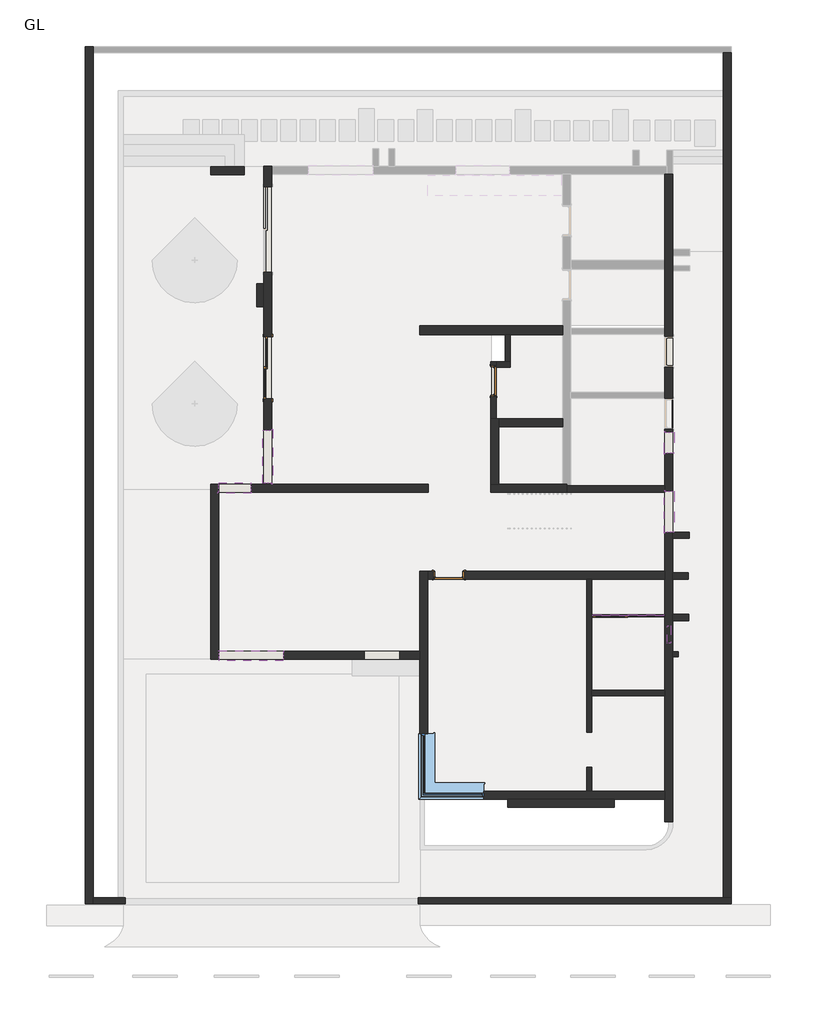
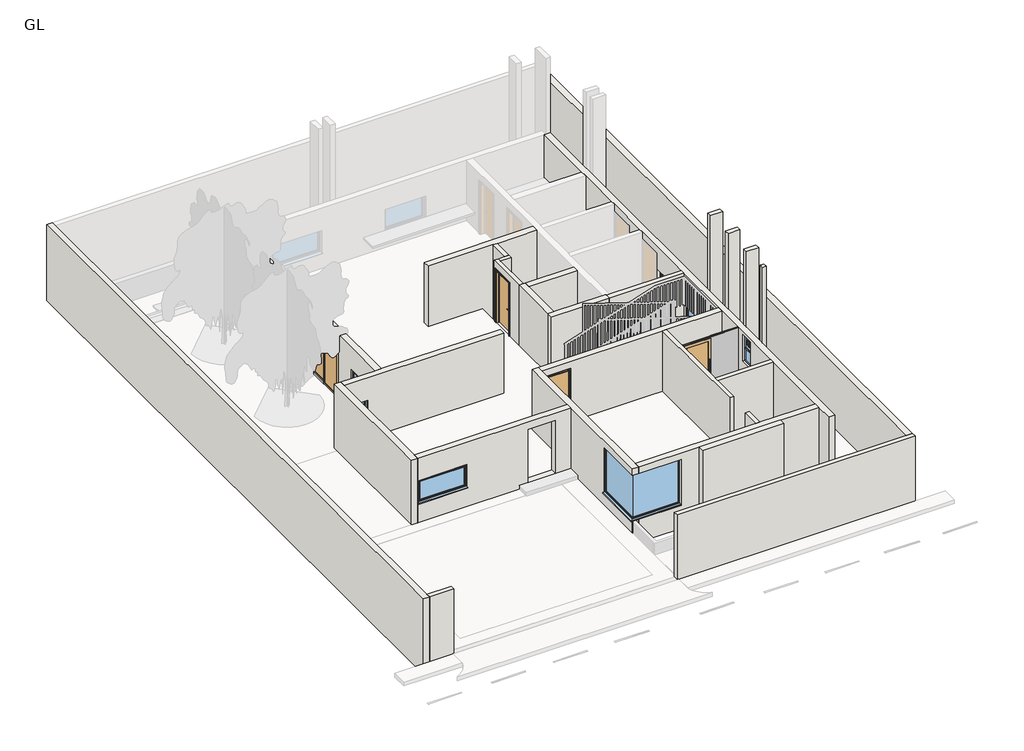
# One storey, part 1 of 6: 30 walls, 7 members, 7 windows, 4 doors, 1 plate.
"""IFC4 building model written with IfcOpenShell, lengths in millimetres."""

from ifc_helpers import new_model, si_unit, point, frame, frame_2d, origin, origin_with_axes, place, context, project, spatial, polyline, circle_curve, ellipse_curve, trimmed, segment, composite_curve, outline, extrude, faceted_brep, transform, mapped, element, save
from ifc_brep_helpers import plane_surface, cylinder_surface, revolved_surface, advanced_brep
from components import door_510b0506, door_61435f0d, door_526ed47c, doors_sgl_glass_1_glass_panel_12mm_thickness_6ba6481b, rectangular_mullion_30mm_square_d725415c, rectangular_mullion_30mm_square_ff288ed3, rectangular_mullion_30mm_square_6919c9ce, system_panel_glazed_4603f3ec, windows_corner_1829x1829mm_2_98ac2af9, windows_sgl_plain_2_8d1346b0, windows_sgl_plain_3_28d0678b, window_6a333e19, windows_sgl_plain_5_79f17ecf, windows_sgl_plain_6_3dcb7f7b

model = new_model("IFC4")

# Units and contexts
model_context = context("Model", 3, world=origin())
ifc_project = project(units=[si_unit("LENGTHUNIT", "METRE", prefix="MILLI")], contexts=[model_context])

# Site, building, storey
site = spatial("IfcSite", under=ifc_project)
building = spatial("IfcBuilding", under=site)
storey = spatial("IfcBuildingStorey", under=building, Name="GL", Elevation=0.0)

# Doors
placement = place(None, origin())
door_shape = door_510b0506(model_context)
element("IfcDoor", 1, ObjectType="5'10\"", at=placement, inside=storey, context=model_context, shape_type="MappedRepresentation", body=[
    mapped(door_shape, transform((-46875.1786333, 21413.0648243, 449.9570313), x_axis=(0.0, 1.0, 0.0), y_axis=(-1.0, 0.0, 0.0), z_axis=(0.0, 0.0, 1.0))),
])
door_2_shape = door_61435f0d(model_context)
element("IfcDoor", 2, ObjectType="Doors_IntSgl : 2'11\"", at=placement, inside=storey, context=model_context, shape_type="MappedRepresentation", body=[
    mapped(door_2_shape, transform((-41829.89796, 15488.6041063, 580.01875), x_axis=(-1.0, 0.0, 0.0), y_axis=(0.0, -1.0, 0.0), z_axis=(0.0, 0.0, 1.0))),
])
door_3_shape = door_526ed47c(model_context)
element("IfcDoor", 3, ObjectType="Doors_IntSgl : 2'11\"", at=placement, inside=storey, context=model_context, shape_type="MappedRepresentation", body=[
    mapped(door_3_shape, transform((-40553.54796, 21038.5041063, 589.9546875), x_axis=(0.0, 1.0, 0.0), y_axis=(-1.0, 0.0, 0.0), z_axis=(0.0, 0.0, 1.0))),
])
doors_sgl_glass_1_glass_panel_12mm_thickness_shape = doors_sgl_glass_1_glass_panel_12mm_thickness_6ba6481b(model_context)
element("IfcDoor", 4, ObjectType="Doors_Sgl_Glass_1 : Glass_Panel-12mm_Thickness", at=placement, inside=storey, context=model_context, shape_type="MappedRepresentation", body=[
    mapped(doors_sgl_glass_1_glass_panel_12mm_thickness_shape, transform((-37210.5680043, 14342.1489352, 629.9757812), x_axis=(-1.0, 0.0, 0.0), y_axis=(0.0, -1.0, 0.0), z_axis=(0.0, 0.0, 1.0))),
])

# Members
rectangular_mullion_30mm_square_shape = rectangular_mullion_30mm_square_d725415c(model_context)
element("IfcMember", 5, ObjectType="Rectangular Mullion : 30mm_Square", at=placement, inside=storey, context=model_context, shape_type="MappedRepresentation", body=[
    mapped(rectangular_mullion_30mm_square_shape, transform((-37710.3080191, 14342.1489352, 3000.0), x_axis=(0.0, 0.0, 1.0), y_axis=(0.0, 1.0, 0.0), z_axis=(-1.0, 0.0, 0.0))),
])
element("IfcMember", 6, ObjectType="Rectangular Mullion : 30mm_Square", at=placement, inside=storey, context=model_context, shape_type="MappedRepresentation", body=[
    mapped(rectangular_mullion_30mm_square_shape, transform((-36680.8279896, 14342.1489352, 3000.0), x_axis=(0.0, 0.0, 1.0), y_axis=(0.0, 1.0, 0.0), z_axis=(-1.0, 0.0, 0.0))),
])
element("IfcMember", 7, ObjectType="Rectangular Mullion : 30mm_Square", at=placement, inside=storey, context=model_context, shape_type="MappedRepresentation", body=[
    mapped(rectangular_mullion_30mm_square_shape, transform((-35681.34796, 14342.1489352, 599.9757812), x_axis=(0.0, 0.0, -1.0), y_axis=(0.0, 1.0, 0.0), z_axis=(1.0, 0.0, 0.0))),
])
element("IfcMember", 8, ObjectType="Rectangular Mullion : 30mm_Square", at=placement, inside=storey, context=model_context, shape_type="MappedRepresentation", body=[
    mapped(rectangular_mullion_30mm_square_shape, transform((-36710.8279896, 14342.1489352, 599.9757812), x_axis=(0.0, 0.0, -1.0), y_axis=(0.0, 1.0, 0.0), z_axis=(1.0, 0.0, 0.0))),
])
rectangular_mullion_30mm_square_2_shape = rectangular_mullion_30mm_square_ff288ed3(model_context)
element("IfcMember", 9, ObjectType="Rectangular Mullion : 30mm_Square", at=placement, inside=storey, context=model_context, shape_type="MappedRepresentation", body=[
    mapped(rectangular_mullion_30mm_square_2_shape, transform((-36695.8279896, 14342.1489352, 599.9757812), x_axis=(-1.0, 0.0, 0.0), y_axis=(0.0, 1.0, 0.0), z_axis=(0.0, 0.0, -1.0))),
])
rectangular_mullion_30mm_square_3_shape = rectangular_mullion_30mm_square_6919c9ce(model_context)
element("IfcMember", 10, ObjectType="Rectangular Mullion : 30mm_Square", at=placement, inside=storey, context=model_context, shape_type="MappedRepresentation", body=[
    mapped(rectangular_mullion_30mm_square_3_shape, transform((-35651.34796, 14342.1489352, 3000.0), x_axis=(1.0, 0.0, 0.0), y_axis=(0.0, 1.0, 0.0), z_axis=(0.0, 0.0, 1.0))),
])
element("IfcMember", 11, ObjectType="Rectangular Mullion : 30mm_Square", at=placement, inside=storey, context=model_context, shape_type="MappedRepresentation", body=[
    mapped(rectangular_mullion_30mm_square_3_shape, transform((-37740.3080191, 14342.1489352, 599.9757812), x_axis=(-1.0, 0.0, 0.0), y_axis=(0.0, 1.0, 0.0), z_axis=(0.0, 0.0, -1.0))),
])

# Plate
system_panel_glazed_shape = system_panel_glazed_4603f3ec(model_context)
element("IfcPlate", 12, ObjectType="System Panel : Glazed", at=placement, inside=storey, context=model_context, shape_type="MappedRepresentation", body=[
    mapped(system_panel_glazed_shape, transform((-36173.5879748, 14342.1489352, 599.9757812), x_axis=(-1.0, 0.0, 0.0), y_axis=(0.0, -1.0, 0.0), z_axis=(0.0, 0.0, 1.0))),
])

# Walls
element("IfcWall", 13, ObjectType="6\" WALL", at=placement, inside=storey, context=model_context, shape_type="SweptSolid", body=[
    extrude(outline(polyline([(-37740.3080191, 9995.8541063), (-37740.3080191, 9303.7041063), (-37892.7080191, 9303.7041063), (-37892.7080191, 9995.8541063), (-37740.3080191, 9995.8541063)])), origin_with_axes(), (0.0, 0.0, 1.0), 3000.0),
])
element("IfcWall", 14, ObjectType="6\" WALL", at=placement, inside=storey, context=model_context, shape_type="Brep", body=[
    faceted_brep([(-37740.3080191, 10999.1541063, 0.0), (-37740.3080191, 12046.9041063, 0.0), (-37740.3080191, 12199.3041063, 0.0), (-37740.3080191, 15374.3041063, 0.0), (-37740.3080191, 15374.3041063, 3000.0), (-37740.3080191, 12199.3041063, 3000.0), (-37740.3080191, 12046.9041063, 3000.0), (-37740.3080191, 10999.1541063, 3000.0), (-37892.7080191, 10999.1541063, 0.0), (-37892.7080191, 10999.1541063, 3000.0), (-37892.7080191, 15374.3041063, 3000.0), (-37892.7080191, 15374.3041063, 0.0)], [[[0, 1, 2, 3, 4, 5, 6, 7]], [[8, 9, 10, 11]], [[3, 2, 1, 0, 8, 11]], [[7, 6, 5, 4, 10, 9]], [[0, 7, 9, 8]], [[4, 3, 11, 10]]]),
])
element("IfcWall", 15, ObjectType="6\" WALL", at=placement, inside=storey, context=model_context, shape_type="Brep", body=[
    faceted_brep([(-40477.34796, 19959.0041063, 0.0), (-40477.34796, 21432.2041063, 0.0), (-40477.34796, 21584.6041063, 0.0), (-40477.34796, 21584.6041063, 3000.0), (-40477.34796, 21432.2041063, 3000.0), (-40477.34796, 19959.0041063, 3000.0), (-40477.34796, 21483.0041063, 2699.9546875), (-40477.34796, 21483.0041063, 589.9546875), (-40477.34796, 20594.0041063, 589.9546875), (-40477.34796, 20594.0041063, 2699.9546875), (-40629.74796, 21584.6041063, 0.0), (-40629.74796, 19959.0041063, 0.0), (-40629.74796, 19959.0041063, 3000.0), (-40629.74796, 21584.6041063, 3000.0), (-40629.74796, 21483.0041063, 589.9546875), (-40629.74796, 21483.0041063, 2699.9546875), (-40629.74796, 20594.0041063, 2699.9546875), (-40629.74796, 20594.0041063, 589.9546875)], [[[0, 1, 2, 3, 4, 5], [6, 7, 8, 9]], [[10, 11, 12, 13], [14, 15, 16, 17]], [[2, 1, 0, 11, 10]], [[5, 4, 3, 13, 12]], [[0, 5, 12, 11]], [[3, 2, 10, 13]], [[14, 7, 6, 15]], [[15, 6, 9, 16]], [[16, 9, 8, 17]], [[7, 14, 17, 8]]]),
])
element("IfcWall", 16, ObjectType="6\" WALL", at=placement, inside=storey, context=model_context, shape_type="Brep", body=[
    faceted_brep([(-40477.34796, 21432.2041063, 0.0), (-40070.94796, 21432.2041063, 0.0), (-40070.94796, 21432.2041063, 3000.0), (-40477.34796, 21432.2041063, 3000.0), (-40477.34796, 21584.6041063, 0.0), (-40477.34796, 21584.6041063, 3000.0), (-40223.34796, 21584.6041063, 3000.0), (-40070.94796, 21584.6041063, 3000.0), (-40070.94796, 21584.6041063, 0.0), (-40223.34796, 21584.6041063, 0.0)], [[[0, 1, 2, 3]], [[4, 5, 6, 7, 8, 9]], [[1, 0, 4, 9, 8]], [[3, 2, 7, 6, 5]], [[0, 3, 5, 4]], [[2, 1, 8, 7]]]),
])
element("IfcWall", 17, ObjectType="6\" WALL", at=placement, inside=storey, context=model_context, shape_type="SweptSolid", body=[
    extrude(outline(polyline([(-40070.94796, 22359.3041063), (-40070.94796, 21584.6041063), (-40223.34796, 21584.6041063), (-40223.34796, 22359.3041063), (-40070.94796, 22359.3041063)])), origin_with_axes(), (0.0, 0.0, 1.0), 3000.0),
])
element("IfcWall", 18, ObjectType="6\" WALL", at=placement, inside=storey, context=model_context, shape_type="SweptSolid", body=[
    extrude(outline(polyline([(-37740.3080191, 12199.3041063), (-35651.34796, 12199.3041063), (-35651.34796, 12046.9041063), (-37740.3080191, 12046.9041063), (-37740.3080191, 12199.3041063)])), origin_with_axes(), (0.0, 0.0, 1.0), 3000.0),
])
element("IfcWall", 19, ObjectType="6\" WALL", at=placement, inside=storey, context=model_context, shape_type="SweptSolid", body=[
    extrude(outline(polyline([(-35422.74796, 13303.4981698), (-35276.2981431, 13303.4981698), (-35276.2981431, 13151.0981698), (-35422.74796, 13151.0981698), (-35422.74796, 13303.4981698)])), origin_with_axes(), (0.0, 0.0, 1.0), 6000.0),
])
element("IfcWall", 20, ObjectType="7\" WALL", at=placement, inside=storey, context=model_context, shape_type="Brep", body=[
    faceted_brep([(-35651.34796, 18041.3041063, 0.0), (-38343.74796, 18041.3041063, 0.0), (-38458.04796, 18041.3041063, 0.0), (-38458.04796, 18041.3041063, 3000.0), (-38343.74796, 18041.3041063, 3000.0), (-35651.34796, 18041.3041063, 3000.0), (-35651.34796, 17863.5041063, 0.0), (-35651.34796, 17863.5041063, 3000.0), (-38458.04796, 17863.5041063, 3000.0), (-38458.04796, 17863.5041063, 0.0)], [[[0, 1, 2, 3, 4, 5]], [[6, 7, 8, 9]], [[2, 1, 0, 6, 9]], [[3, 2, 9, 8]], [[5, 4, 3, 8, 7]], [[0, 5, 7, 6]]]),
])
element("IfcWall", 21, ObjectType="7\" WALL", at=placement, inside=storey, context=model_context, shape_type="SweptSolid", body=[
    extrude(outline(polyline([(-51085.1791975, 6088.2065956), (-51999.5791975, 6088.2065956), (-51999.5791975, 6266.0065956), (-51085.1791975, 6266.0065956), (-51085.1791975, 6088.2065956)])), origin_with_axes(), (0.0, 0.0, 1.0), 3000.0),
])
element("IfcWall", 22, ObjectType="7\" WALL", at=placement, inside=storey, context=model_context, shape_type="Brep", body=[
    faceted_brep([(-42703.1791975, 6088.2065956, 0.0), (-33762.3791975, 6088.2065956, 0.0), (-33762.3791975, 6088.2065956, 3000.0), (-42703.1791975, 6088.2065956, 3000.0), (-42703.1791975, 6266.0065956, 0.0), (-42703.1791975, 6266.0065956, 3000.0), (-33990.9791975, 6266.0065956, 3000.0), (-33762.3791975, 6266.0065956, 3000.0), (-33762.3791975, 6266.0065956, 0.0), (-33990.9791975, 6266.0065956, 0.0)], [[[0, 1, 2, 3]], [[4, 5, 6, 7, 8, 9]], [[1, 0, 4, 9, 8]], [[3, 2, 7, 6, 5]], [[0, 3, 5, 4]], [[2, 1, 8, 7]]]),
])
element("IfcWall", 23, ObjectType="7\" WALL", at=placement, inside=storey, context=model_context, shape_type="SweptSolid", body=[
    extrude(outline(polyline([(-35422.74796, 14367.5489352), (-34966.0759444, 14367.5489352), (-34966.0759444, 14189.7489352), (-35422.74796, 14189.7489352), (-35422.74796, 14367.5489352)])), origin_with_axes(), (0.0, 0.0, 1.0), 6000.0),
])
element("IfcWall", 24, ObjectType="7\" WALL", at=placement, inside=storey, context=model_context, shape_type="SweptSolid", body=[
    extrude(outline(polyline([(-35422.74796, 15551.8272539), (-34982.9645404, 15551.8272539), (-34982.9645404, 15374.0272539), (-35422.74796, 15374.0272539), (-35422.74796, 15551.8272539)])), origin_with_axes(), (0.0, 0.0, 1.0), 6000.0),
])
element("IfcWall", 25, ObjectType="7\" WALL", at=placement, inside=storey, context=model_context, shape_type="SweptSolid", body=[
    extrude(outline(polyline([(-35422.74796, 16715.1290984), (-34962.7027512, 16715.1290984), (-34962.7027512, 16537.3290984), (-35422.74796, 16537.3290984), (-35422.74796, 16715.1290984)])), origin_with_axes(), (0.0, 0.0, 1.0), 6000.0),
])
element("IfcWall", 26, ObjectType="8\" WALL", at=placement, inside=storey, context=model_context, shape_type="SweptSolid", body=[
    extrude(outline(polyline([(-47318.6226721, 23155.7652167), (-47318.6226721, 23816.1652167), (-47115.4226721, 23816.1652167), (-47115.4226721, 23155.7652167), (-47318.6226721, 23155.7652167)])), origin_with_axes(), (0.0, 0.0, 1.0), 3000.0),
])
element("IfcWall", 27, ObjectType="9\" INNER WALL", at=placement, inside=storey, context=model_context, shape_type="Brep", body=[
    faceted_brep([(-48411.8786333, 18085.6648243, 0.0), (-48411.8786333, 18085.6648243, 1200.0), (-47497.4786333, 18085.6648243, 1200.0), (-47497.4786333, 18085.6648243, 2110.0), (-48411.8786333, 18085.6648243, 2110.0), (-48411.8786333, 18085.6648243, 3000.0), (-47116.4786333, 18085.6648243, 3000.0), (-46887.8786333, 18085.6648243, 3000.0), (-42417.4786333, 18085.6648243, 3000.0), (-42417.4786333, 18085.6648243, 0.0), (-46887.8786333, 18085.6648243, 0.0), (-47116.4786333, 18085.6648243, 0.0), (-47497.4786333, 17857.0648243, 1200.0), (-48411.8786333, 17857.0648243, 1200.0), (-48411.8786333, 17857.0648243, 0.0), (-42417.4786333, 17857.0648243, 0.0), (-42417.4786333, 17857.0648243, 3000.0), (-48411.8786333, 17857.0648243, 3000.0), (-48411.8786333, 17857.0648243, 2110.0), (-47497.4786333, 17857.0648243, 2110.0)], [[[0, 1, 2, 3, 4, 5, 6, 7, 8, 9, 10, 11]], [[12, 13, 14, 15, 16, 17, 18, 19]], [[0, 11, 10, 9, 15, 14]], [[8, 7, 6, 5, 17, 16]], [[9, 8, 16, 15]], [[18, 17, 5, 4]], [[14, 13, 1, 0]], [[2, 1, 13, 12]], [[3, 2, 12, 19]], [[4, 3, 19, 18]]]),
])
element("IfcWall", 28, ObjectType="9\" INNER WALL", at=placement, inside=storey, context=model_context, shape_type="Brep", body=[
    faceted_brep([(-48640.4786333, 18085.6648243, 0.0), (-48640.4786333, 13078.7799463, 0.0), (-48640.4786333, 13078.7799463, 3000.0), (-48640.4786333, 18085.6648243, 3000.0), (-48411.8786333, 18085.6648243, 0.0), (-48411.8786333, 18085.6648243, 3000.0), (-48411.8786333, 17857.0648243, 3000.0), (-48411.8786333, 13307.3799463, 3000.0), (-48411.8786333, 13078.7799463, 3000.0), (-48411.8786333, 13078.7799463, 0.0), (-48411.8786333, 13307.3799463, 0.0), (-48411.8786333, 17857.0648243, 0.0)], [[[0, 1, 2, 3]], [[4, 5, 6, 7, 8, 9, 10, 11]], [[1, 0, 4, 11, 10, 9]], [[3, 2, 8, 7, 6, 5]], [[0, 3, 5, 4]], [[2, 1, 9, 8]]]),
])
element("IfcWall", 29, ObjectType="9\" INNER WALL", at=placement, inside=storey, context=model_context, shape_type="Brep", body=[
    faceted_brep([(-46887.8786333, 18085.6648243, 0.0), (-46887.8786333, 26943.9148243, 0.0), (-46887.8786333, 27172.5148243, 0.0), (-46887.8786333, 27172.5148243, 3000.0), (-46887.8786333, 26943.9148243, 3000.0), (-46887.8786333, 18085.6648243, 3000.0), (-46887.8786333, 18111.0648243, 2110.0), (-46887.8786333, 19635.0648243, 2110.0), (-46887.8786333, 19635.0648243, 1200.0), (-46887.8786333, 18111.0648243, 1200.0), (-46887.8786333, 20524.0648243, 2583.9570312), (-46887.8786333, 22302.0648243, 2583.9570312), (-46887.8786333, 22302.0648243, 449.9570312), (-46887.8786333, 20524.0648243, 449.9570313), (-46887.8786333, 24149.9148243, 2583.9570312), (-46887.8786333, 26588.3148243, 2583.9570312), (-46887.8786333, 26588.3148243, 449.9570312), (-46887.8786333, 24149.9148243, 449.9570313), (-47116.4786333, 18085.6648243, 0.0), (-47116.4786333, 18085.6648243, 3000.0), (-47116.4786333, 27172.5148243, 3000.0), (-47116.4786333, 27172.5148243, 0.0), (-47116.4786333, 18111.0648243, 2110.0), (-47116.4786333, 18111.0648243, 1200.0), (-47116.4786333, 19635.0648243, 1200.0), (-47116.4786333, 19635.0648243, 2110.0), (-47116.4786333, 20524.0648243, 2583.9570312), (-47116.4786333, 20524.0648243, 449.9570313), (-47116.4786333, 22302.0648243, 449.9570313), (-47116.4786333, 22302.0648243, 2583.9570312), (-47116.4786333, 24149.9148243, 2583.9570312), (-47116.4786333, 24149.9148243, 449.9570313), (-47116.4786333, 26588.3148243, 449.9570313), (-47116.4786333, 26588.3148243, 2583.9570312)], [[[0, 1, 2, 3, 4, 5], [6, 7, 8, 9], [10, 11, 12, 13], [14, 15, 16, 17]], [[18, 19, 20, 21], [22, 23, 24, 25], [26, 27, 28, 29], [30, 31, 32, 33]], [[2, 1, 0, 18, 21]], [[5, 4, 3, 20, 19]], [[0, 5, 19, 18]], [[3, 2, 21, 20]], [[23, 22, 6, 9]], [[24, 23, 9, 8]], [[25, 24, 8, 7]], [[22, 25, 7, 6]], [[27, 26, 10, 13]], [[28, 27, 13, 12]], [[29, 28, 12, 11]], [[26, 29, 11, 10]], [[31, 30, 14, 17]], [[32, 31, 17, 16]], [[33, 32, 16, 15]], [[30, 33, 15, 14]]]),
])
element("IfcWall", 30, ObjectType="9\" INNER WALL", at=placement, inside=storey, context=model_context, shape_type="SweptSolid", body=[
    extrude(outline(polyline([(0.0, -48411.8786333), (0.0, -42655.39796), (3000.0, -42655.39796), (3000.0, -48411.8786333), (0.0, -48411.8786333)]), holes=[polyline([(2709.9757813, -44249.59796), (2709.9757813, -43239.59796), (599.9757812, -43239.59796), (599.9757812, -44249.59796), (2709.9757813, -44249.59796)]), polyline([(2110.0, -48386.4786333), (2110.0, -46557.6786333), (1200.0, -46557.6786333), (1200.0, -48386.4786333), (2110.0, -48386.4786333)])]), frame((0.0, 13078.7799463, 0.0), z_axis=(0.0, 1.0, 0.0), x_axis=(0.0, 0.0, 1.0)), (0.0, 0.0, 1.0), 228.6),
])
element("IfcWall", 31, ObjectType="9\" INNER WALL", at=placement, inside=storey, context=model_context, shape_type="Brep", body=[
    faceted_brep([(-42655.39796, 15602.9041063, 0.0), (-42655.39796, 13307.3799463, 0.0), (-42655.39796, 13078.7799463, 0.0), (-42655.39796, 9075.1041063, 0.0), (-42655.39796, 9075.1041063, 914.4), (-42655.39796, 10950.9041063, 914.4), (-42655.39796, 10950.9041063, 2743.2), (-42655.39796, 9075.1041063, 2743.2), (-42655.39796, 9075.1041063, 3000.0), (-42655.39796, 13078.7799463, 3000.0), (-42655.39796, 13307.3799463, 3000.0), (-42655.39796, 15602.9041063, 3000.0), (-42426.79796, 9075.1041063, 0.0), (-42426.79796, 9303.7041063, 0.0), (-42426.79796, 15374.3041063, 0.0), (-42426.79796, 15602.9041063, 0.0), (-42426.79796, 15602.9041063, 3000.0), (-42426.79796, 15374.3041063, 3000.0), (-42426.79796, 9303.7041063, 3000.0), (-42426.79796, 9075.1041063, 3000.0), (-42426.79796, 9075.1041063, 2743.2), (-42426.79796, 9303.7041063, 2743.2), (-42426.79796, 9547.1041063, 2743.2), (-42426.79796, 10950.9041063, 2743.2), (-42426.79796, 10950.9041063, 914.4), (-42426.79796, 9547.1041063, 914.4), (-42426.79796, 9303.7041063, 914.4), (-42426.79796, 9075.1041063, 914.4)], [[[0, 1, 2, 3, 4, 5, 6, 7, 8, 9, 10, 11]], [[12, 13, 14, 15, 16, 17, 18, 19, 20, 21, 22, 23, 24, 25, 26, 27]], [[3, 2, 1, 0, 15, 14, 13, 12]], [[11, 10, 9, 8, 19, 18, 17, 16]], [[3, 12, 27, 4]], [[19, 8, 7, 20]], [[0, 11, 16, 15]], [[6, 23, 22, 21, 20, 7]], [[24, 5, 4, 27, 26, 25]], [[23, 6, 5, 24]]]),
])
element("IfcWall", 32, ObjectType="9\" INNER WALL", at=placement, inside=storey, context=model_context, shape_type="Brep", body=[
    faceted_brep([(-42426.79796, 9075.1041063, 0.0), (-35651.34796, 9075.1041063, 0.0), (-35651.34796, 9075.1041063, 3000.0), (-42426.79796, 9075.1041063, 3000.0), (-42426.79796, 9075.1041063, 2743.2), (-40826.59796, 9075.1041063, 2743.2), (-40826.59796, 9075.1041063, 914.4), (-42426.79796, 9075.1041063, 914.4), (-35651.34796, 9303.7041063, 0.0), (-37740.3080191, 9303.7041063, 0.0), (-37892.7080191, 9303.7041063, 0.0), (-42426.79796, 9303.7041063, 0.0), (-42426.79796, 9303.7041063, 914.4), (-40826.59796, 9303.7041063, 914.4), (-40826.59796, 9303.7041063, 2743.2), (-42426.79796, 9303.7041063, 2743.2), (-42426.79796, 9303.7041063, 3000.0), (-37892.7080191, 9303.7041063, 3000.0), (-37740.3080191, 9303.7041063, 3000.0), (-35651.34796, 9303.7041063, 3000.0)], [[[0, 1, 2, 3, 4, 5, 6, 7]], [[8, 9, 10, 11, 12, 13, 14, 15, 16, 17, 18, 19]], [[1, 0, 11, 10, 9, 8]], [[3, 2, 19, 18, 17, 16]], [[3, 16, 15, 4]], [[11, 0, 7, 12]], [[2, 1, 8, 19]], [[14, 5, 4, 15]], [[6, 13, 12, 7]], [[5, 14, 13, 6]]]),
])
element("IfcWall", 33, ObjectType="9\" INNER WALL", at=placement, inside=storey, context=model_context, shape_type="Brep", body=[
    faceted_brep([(-35422.74796, 8440.1041063, 0.0), (-35422.74796, 13151.0981698, 0.0), (-35422.74796, 13303.4981698, 0.0), (-35422.74796, 14189.7489352, 0.0), (-35422.74796, 14367.5489352, 0.0), (-35422.74796, 15374.0272539, 0.0), (-35422.74796, 15551.8272539, 0.0), (-35422.74796, 16537.3290984, 0.0), (-35422.74796, 16715.1290984, 0.0), (-35422.74796, 24184.7254786, 0.0), (-35422.74796, 24337.1254786, 0.0), (-35422.74796, 24619.9041063, 0.0), (-35422.74796, 24797.7041063, 0.0), (-35422.74796, 26943.9148243, 0.0), (-35422.74796, 26943.9148243, 3000.0), (-35422.74796, 8440.1041063, 3000.0), (-35422.74796, 13537.3489352, 1828.8), (-35422.74796, 13537.3489352, 2878.8), (-35422.74796, 14037.3489352, 2878.8), (-35422.74796, 14037.3489352, 1828.8), (-35422.74796, 20543.2041063, 2699.9546875), (-35422.74796, 20543.2041063, 589.9546875), (-35422.74796, 19654.2041063, 589.9546875), (-35422.74796, 19654.2041063, 2699.9546875), (-35422.74796, 22321.2041063, 2699.9546875), (-35422.74796, 22321.2041063, 589.9546875), (-35422.74796, 21432.2041063, 589.9546875), (-35422.74796, 21432.2041063, 2699.9546875), (-35422.74796, 17883.5290984, 2110.0), (-35422.74796, 17883.5290984, 1200.0), (-35422.74796, 16715.1290984, 1200.0), (-35422.74796, 16715.1290984, 2110.0), (-35422.74796, 19578.0041063, 2110.0), (-35422.74796, 19578.0041063, 1200.0), (-35422.74796, 18968.4041063, 1200.0), (-35422.74796, 18968.4041063, 2110.0), (-35651.34796, 26943.9148243, 0.0), (-35651.34796, 24492.9041063, 0.0), (-35651.34796, 24238.9041063, 0.0), (-35651.34796, 22549.8041063, 0.0), (-35651.34796, 22372.0041063, 0.0), (-35651.34796, 20721.0041063, 0.0), (-35651.34796, 20543.2041063, 0.0), (-35651.34796, 18041.3041063, 0.0), (-35651.34796, 17863.5041063, 0.0), (-35651.34796, 15602.9041063, 0.0), (-35651.34796, 15374.3041063, 0.0), (-35651.34796, 12199.3041063, 0.0), (-35651.34796, 12046.9041063, 0.0), (-35651.34796, 9303.7041063, 0.0), (-35651.34796, 9075.1041063, 0.0), (-35651.34796, 8440.1041063, 0.0), (-35651.34796, 8440.1041063, 3000.0), (-35651.34796, 9075.1041063, 3000.0), (-35651.34796, 9303.7041063, 3000.0), (-35651.34796, 12046.9041063, 3000.0), (-35651.34796, 12199.3041063, 3000.0), (-35651.34796, 15374.3041063, 3000.0), (-35651.34796, 15602.9041063, 3000.0), (-35651.34796, 17863.5041063, 3000.0), (-35651.34796, 18041.3041063, 3000.0), (-35651.34796, 20543.2041063, 3000.0), (-35651.34796, 20721.0041063, 3000.0), (-35651.34796, 22372.0041063, 3000.0), (-35651.34796, 22549.8041063, 3000.0), (-35651.34796, 24238.9041063, 3000.0), (-35651.34796, 24492.9041063, 3000.0), (-35651.34796, 26943.9148243, 3000.0), (-35651.34796, 13537.3489352, 2878.8), (-35651.34796, 13537.3489352, 1828.8), (-35651.34796, 14037.3489352, 1828.8), (-35651.34796, 14037.3489352, 2878.8), (-35651.34796, 20543.2041063, 589.9546875), (-35651.34796, 20543.2041063, 2699.9546875), (-35651.34796, 19654.2041063, 2699.9546875), (-35651.34796, 19654.2041063, 589.9546875), (-35651.34796, 22321.2041063, 589.9546875), (-35651.34796, 22321.2041063, 2699.9546875), (-35651.34796, 21432.2041063, 2699.9546875), (-35651.34796, 21432.2041063, 589.9546875), (-35651.34796, 17883.5290984, 2110.0), (-35651.34796, 16715.1290984, 2110.0), (-35651.34796, 16715.1290984, 1200.0), (-35651.34796, 17883.5290984, 1200.0), (-35651.34796, 19578.0041063, 2110.0), (-35651.34796, 18968.4041063, 2110.0), (-35651.34796, 18968.4041063, 1200.0), (-35651.34796, 19578.0041063, 1200.0), (-35600.54796, 26943.9148243, 0.0), (-35600.54796, 26943.9148243, 3000.0)], [[[0, 1, 2, 3, 4, 5, 6, 7, 8, 9, 10, 11, 12, 13, 14, 15], [16, 17, 18, 19], [20, 21, 22, 23], [24, 25, 26, 27], [28, 29, 30, 31], [32, 33, 34, 35]], [[36, 37, 38, 39, 40, 41, 42, 43, 44, 45, 46, 47, 48, 49, 50, 51, 52, 53, 54, 55, 56, 57, 58, 59, 60, 61, 62, 63, 64, 65, 66, 67], [68, 69, 70, 71], [72, 73, 74, 75], [76, 77, 78, 79], [80, 81, 82, 83], [84, 85, 86, 87]], [[13, 12, 11, 10, 9, 8, 7, 6, 5, 4, 3, 2, 1, 0, 51, 50, 49, 48, 47, 46, 45, 44, 43, 42, 41, 40, 39, 38, 37, 36, 88]], [[15, 14, 89, 67, 66, 65, 64, 63, 62, 61, 60, 59, 58, 57, 56, 55, 54, 53, 52]], [[0, 15, 52, 51]], [[14, 13, 88, 36, 67, 89]], [[69, 68, 17, 16]], [[70, 69, 16, 19]], [[71, 70, 19, 18]], [[68, 71, 18, 17]], [[72, 21, 20, 73]], [[73, 20, 23, 74]], [[74, 23, 22, 75]], [[21, 72, 75, 22]], [[76, 25, 24, 77]], [[77, 24, 27, 78]], [[26, 79, 78, 27]], [[25, 76, 79, 26]], [[29, 28, 80, 83]], [[30, 29, 83, 82]], [[31, 30, 82, 81]], [[28, 31, 81, 80]], [[33, 32, 84, 87]], [[34, 33, 87, 86]], [[35, 34, 86, 85]], [[32, 35, 85, 84]]]),
])
element("IfcWall", 34, ObjectType="9\" INNER WALL", at=placement, inside=storey, context=model_context, shape_type="Brep", body=[
    faceted_brep([(-42426.79796, 15374.3041063, 0.0), (-37892.7080191, 15374.3041063, 0.0), (-37740.3080191, 15374.3041063, 0.0), (-35651.34796, 15374.3041063, 0.0), (-35651.34796, 15374.3041063, 3000.0), (-37740.3080191, 15374.3041063, 3000.0), (-37892.7080191, 15374.3041063, 3000.0), (-42426.79796, 15374.3041063, 3000.0), (-42274.39796, 15374.3041063, 580.01875), (-42274.39796, 15374.3041063, 2690.01875), (-41385.39796, 15374.3041063, 2690.01875), (-41385.39796, 15374.3041063, 580.01875), (-42426.79796, 15602.9041063, 0.0), (-42426.79796, 15602.9041063, 3000.0), (-35651.34796, 15602.9041063, 3000.0), (-35651.34796, 15602.9041063, 0.0), (-42274.39796, 15602.9041063, 580.01875), (-41385.39796, 15602.9041063, 580.01875), (-41385.39796, 15602.9041063, 2690.01875), (-42274.39796, 15602.9041063, 2690.01875)], [[[0, 1, 2, 3, 4, 5, 6, 7], [8, 9, 10, 11]], [[12, 13, 14, 15], [16, 17, 18, 19]], [[3, 2, 1, 0, 12, 15]], [[7, 6, 5, 4, 14, 13]], [[0, 7, 13, 12]], [[4, 3, 15, 14]], [[9, 8, 16, 19]], [[10, 9, 19, 18]], [[11, 10, 18, 17]], [[8, 11, 17, 16]]]),
])
element("IfcWall", 35, ObjectType="9\" INNER WALL", at=placement, inside=storey, context=model_context, shape_type="Brep", body=[
    faceted_brep([(-38458.04796, 18092.1041063, 0.0), (-38572.34796, 18092.1041063, 0.0), (-40401.14796, 18092.1041063, 0.0), (-40629.74796, 18092.1041063, 0.0), (-40629.74796, 18092.1041063, 3000.0), (-40401.14796, 18092.1041063, 3000.0), (-38572.34796, 18092.1041063, 3000.0), (-38458.04796, 18092.1041063, 3000.0), (-38458.04796, 17863.5041063, 0.0), (-38458.04796, 17863.5041063, 3000.0), (-40629.74796, 17863.5041063, 3000.0), (-40629.74796, 17863.5041063, 0.0), (-38458.04796, 18041.3041063, 0.0), (-38458.04796, 18041.3041063, 3000.0)], [[[0, 1, 2, 3, 4, 5, 6, 7]], [[8, 9, 10, 11]], [[3, 2, 1, 0, 12, 8, 11]], [[7, 6, 5, 4, 10, 9, 13]], [[0, 7, 13, 9, 8, 12]], [[4, 3, 11, 10]]]),
])
element("IfcWall", 36, ObjectType="9\" INNER WALL", at=placement, inside=storey, context=model_context, shape_type="Brep", body=[
    faceted_brep([(-40401.14796, 18092.1041063, 0.0), (-40401.14796, 19730.4041063, 0.0), (-40401.14796, 19959.0041063, 0.0), (-40401.14796, 19959.0041063, 3000.0), (-40401.14796, 19730.4041063, 3000.0), (-40401.14796, 18092.1041063, 3000.0), (-40629.74796, 18092.1041063, 0.0), (-40629.74796, 18092.1041063, 3000.0), (-40629.74796, 19959.0041063, 3000.0), (-40629.74796, 19959.0041063, 0.0), (-40477.34796, 19959.0041063, 0.0), (-40477.34796, 19959.0041063, 3000.0)], [[[0, 1, 2, 3, 4, 5]], [[6, 7, 8, 9]], [[2, 1, 0, 6, 9, 10]], [[5, 4, 3, 11, 8, 7]], [[0, 5, 7, 6]], [[3, 2, 10, 9, 8, 11]]]),
])
element("IfcWall", 37, ObjectType="9\" INNER WALL", at=placement, inside=storey, context=model_context, shape_type="SweptSolid", body=[
    extrude(outline(polyline([(-38572.34796, 19730.4041063), (-40401.14796, 19730.4041063), (-40401.14796, 19959.0041063), (-38572.34796, 19959.0041063), (-38572.34796, 19730.4041063)])), origin_with_axes(), (0.0, 0.0, 1.0), 3000.0),
])
element("IfcWall", 38, ObjectType="9\" INNER WALL", at=placement, inside=storey, context=model_context, shape_type="Brep", body=[
    faceted_brep([(-52228.1791975, 30599.2065956, 0.0), (-52228.1791975, 6088.2065956, 0.0), (-52228.1791975, 6088.2065956, 3000.0), (-52228.1791975, 30599.2065956, 3000.0), (-51999.5791975, 30599.2065956, 0.0), (-51999.5791975, 30599.2065956, 3000.0), (-51999.5791975, 30421.4065956, 3000.0), (-51999.5791975, 6266.0065956, 3000.0), (-51999.5791975, 6088.2065956, 3000.0), (-51999.5791975, 6088.2065956, 0.0), (-51999.5791975, 6266.0065956, 0.0), (-51999.5791975, 30421.4065956, 0.0)], [[[0, 1, 2, 3]], [[4, 5, 6, 7, 8, 9, 10, 11]], [[1, 0, 4, 11, 10, 9]], [[3, 2, 8, 7, 6, 5]], [[2, 1, 9, 8]], [[0, 3, 5, 4]]]),
])
element("IfcWall", 39, ObjectType="9\" INNER WALL", at=placement, inside=storey, context=model_context, shape_type="SweptSolid", body=[
    extrude(outline(polyline([(-33990.9791975, 6266.0065956), (-33990.9791975, 30421.4065956), (-33762.3791975, 30421.4065956), (-33762.3791975, 6266.0065956), (-33990.9791975, 6266.0065956)])), origin_with_axes(), (0.0, 0.0, 1.0), 3000.0),
])
element("IfcWall", 40, ObjectType="9\" INNER WALL", at=placement, inside=storey, context=model_context, shape_type="SweptSolid", body=[
    extrude(outline(polyline([(-40146.5645668, 9077.2024337), (-37098.5645668, 9077.2024337), (-37098.5645668, 8848.6024337), (-40146.5645668, 8848.6024337), (-40146.5645668, 9077.2024337)])), origin_with_axes(), (0.0, 0.0, 1.0), 3000.0),
])
element("IfcWall", 41, ObjectType="9\" INNER WALL", at=placement, inside=storey, context=model_context, shape_type="SweptSolid", body=[
    extrude(outline(polyline([(-47681.6286333, 26935.1616741), (-48640.4786333, 26935.1616741), (-48640.4786333, 27163.7616741), (-47681.6286333, 27163.7616741), (-47681.6286333, 26935.1616741)])), origin_with_axes(), (0.0, 0.0, 1.0), 3000.0),
])
element("IfcWall", 42, ObjectType="9\" INNER WALL 2", at=placement, inside=storey, context=model_context, shape_type="Brep", body=[
    faceted_brep([(-38572.34796, 22613.3041063, 0.0), (-42661.74796, 22613.3041063, 0.0), (-42661.74796, 22613.3041063, 3000.0), (-38572.34796, 22613.3041063, 3000.0), (-38572.34796, 22359.3041063, 0.0), (-38572.34796, 22359.3041063, 3000.0), (-40070.94796, 22359.3041063, 3000.0), (-40223.34796, 22359.3041063, 3000.0), (-42661.74796, 22359.3041063, 3000.0), (-42661.74796, 22359.3041063, 0.0), (-40223.34796, 22359.3041063, 0.0), (-40070.94796, 22359.3041063, 0.0)], [[[0, 1, 2, 3]], [[4, 5, 6, 7, 8, 9, 10, 11]], [[1, 0, 4, 11, 10, 9]], [[2, 1, 9, 8]], [[3, 2, 8, 7, 6, 5]], [[0, 3, 5, 4]]]),
])

# Windows
element("IfcWindow", 43, ObjectType="Bathroom-Window-with-Vent_Fan : B", at=placement, inside=storey, context=model_context, shape_type="SolidModel", body=[
    extrude(outline(polyline([(13537.3489352, 1828.8), (13537.3489352, 2878.8), (14037.3489352, 2878.8), (14037.3489352, 1828.8), (13537.3489352, 1828.8)]), holes=[polyline([(13577.3489352, 2838.8), (13577.3489352, 1868.8), (13997.3489352, 1868.8), (13997.3489352, 2838.8), (13577.3489352, 2838.8)])]), frame((-35588.24796, 0.0, 0.0), z_axis=(1.0, 0.0, 0.0), x_axis=(0.0, 1.0, 0.0)), (0.0, 0.0, 1.0), 100.0),
    extrude(outline(polyline([(-35541.24796, 13997.3489352), (-35541.24796, 13577.3489352), (-35553.24796, 13577.3489352), (-35553.24796, 13997.3489352), (-35541.24796, 13997.3489352)])), frame((0.0, 0.0, 1868.8), z_axis=(0.0, 0.0, 1.0), x_axis=(1.0, 0.0, 0.0)), (0.0, 0.0, 1.0), 460.0),
    extrude(outline(composite_curve([segment(polyline([(13877.9797139, 2586.5381738), (13787.3489352, 2623.8), (13696.7181565, 2586.5381738)]), True, "CONTINUOUS"), segment(trimmed(circle_curve(frame_2d((13757.6638179, 2628.8)), 74.1649216), [point((13696.7181565, 2586.5381738))], [point((13696.7181565, 2671.0618262))], False, "CARTESIAN"), True, "CONTINUOUS"), segment(polyline([(13696.7181565, 2671.0618262), (13787.3489352, 2633.8), (13877.9797139, 2671.0618262)]), True, "CONTINUOUS"), segment(trimmed(circle_curve(frame_2d((13817.0340525, 2628.8)), 74.1649216), [point((13877.9797139, 2671.0618262))], [point((13877.9797139, 2586.5381738))], False, "CARTESIAN"), True, "CONTINUOUS")], self_intersect=False)), frame((-35553.24796, 0.0, 0.0), z_axis=(1.0, 0.0, 0.0), x_axis=(0.0, 1.0, 0.0)), (0.0, 0.0, 1.0), 12.0),
    extrude(outline(composite_curve([segment(polyline([(13829.6107614, 2719.4307787), (13792.3489352, 2628.8), (13829.6107614, 2538.1692213)]), True, "CONTINUOUS"), segment(trimmed(circle_curve(frame_2d((13787.3489352, 2599.1148827)), 74.1649216), [point((13829.6107614, 2538.1692213))], [point((13745.087109, 2538.1692213))], False, "CARTESIAN"), True, "CONTINUOUS"), segment(polyline([(13745.087109, 2538.1692213), (13782.3489352, 2628.8), (13745.087109, 2719.4307787)]), True, "CONTINUOUS"), segment(trimmed(circle_curve(frame_2d((13787.3489352, 2658.4851173)), 74.1649216), [point((13745.087109, 2719.4307787))], [point((13829.6107614, 2719.4307787))], False, "CARTESIAN"), True, "CONTINUOUS")], self_intersect=False)), frame((-35553.24796, 0.0, 0.0), z_axis=(1.0, 0.0, 0.0), x_axis=(0.0, 1.0, 0.0)), (0.0, 0.0, 1.0), 12.0),
    advanced_brep(
    [(-35539.24796, 13787.3489352, 2738.7561319), (-35539.24796, 13787.3489352, 2518.8438681), (-35555.24796, 13787.3489352, 2518.8438681), (-35555.24796, 13787.3489352, 2738.7561319), (-35560.24796, 13787.3489352, 2758.7561319), (-35560.24796, 13787.3489352, 2498.8438681), (-35534.24796, 13787.3489352, 2498.8438681), (-35534.24796, 13787.3489352, 2758.7561319), (-35565.24796, 13787.3489352, 2753.7561319), (-35565.24796, 13787.3489352, 2503.8438681), (-35565.24796, 13787.3489352, 2508.8438681), (-35565.24796, 13787.3489352, 2748.7561319), (-35529.24796, 13787.3489352, 2503.8438681), (-35529.24796, 13787.3489352, 2753.7561319), (-35529.24796, 13787.3489352, 2748.7561319), (-35529.24796, 13787.3489352, 2508.8438681)],
    [
        (0, 1, circle_curve(frame((-35539.24796, 13787.3489352, 2628.8), z_axis=(1.0, 0.0, 0.0), x_axis=(0.0, 0.0, -1.0)), 109.9561319)),
        (1, 2),
        (2, 3, circle_curve(frame((-35555.24796, 13787.3489352, 2628.8), z_axis=(-1.0, 0.0, 0.0), x_axis=(0.0, 0.0, -1.0)), 109.9561319)),
        (3, 0),
        (4, 5, circle_curve(frame((-35560.24796, 13787.3489352, 2628.8), z_axis=(1.0, 0.0, 0.0), x_axis=(0.0, 0.0, -1.0)), 129.9561319)),
        (5, 6),
        (6, 7, circle_curve(frame((-35534.24796, 13787.3489352, 2628.8), z_axis=(-1.0, 0.0, 0.0), x_axis=(0.0, 0.0, -1.0)), 129.9561319)),
        (7, 4),
        (8, 9, circle_curve(frame((-35565.24796, 13787.3489352, 2628.8), z_axis=(-1.0, 0.0, 0.0), x_axis=(0.0, 0.0, 1.0)), 124.9561319)),
        (9, 8, circle_curve(frame((-35565.24796, 13787.3489352, 2628.8), z_axis=(-1.0, 0.0, 0.0), x_axis=(0.0, 0.0, -1.0)), 124.9561319)),
        (10, 11, circle_curve(frame((-35565.24796, 13787.3489352, 2628.8), z_axis=(1.0, 0.0, 0.0), x_axis=(0.0, 0.0, 1.0)), 119.9561319)),
        (11, 10, circle_curve(frame((-35565.24796, 13787.3489352, 2628.8), z_axis=(1.0, 0.0, 0.0), x_axis=(0.0, 0.0, -1.0)), 119.9561319)),
        (1, 0, circle_curve(frame((-35539.24796, 13787.3489352, 2628.8), z_axis=(1.0, 0.0, 0.0), x_axis=(0.0, 0.0, 1.0)), 109.9561319)),
        (3, 2, circle_curve(frame((-35555.24796, 13787.3489352, 2628.8), z_axis=(-1.0, 0.0, 0.0), x_axis=(0.0, 0.0, 1.0)), 109.9561319)),
        (12, 13, circle_curve(frame((-35529.24796, 13787.3489352, 2628.8), z_axis=(1.0, 0.0, 0.0), x_axis=(0.0, 0.0, 1.0)), 124.9561319)),
        (13, 12, circle_curve(frame((-35529.24796, 13787.3489352, 2628.8), z_axis=(1.0, 0.0, 0.0), x_axis=(0.0, 0.0, -1.0)), 124.9561319)),
        (14, 15, circle_curve(frame((-35529.24796, 13787.3489352, 2628.8), z_axis=(-1.0, 0.0, 0.0), x_axis=(0.0, 0.0, 1.0)), 119.9561319)),
        (15, 14, circle_curve(frame((-35529.24796, 13787.3489352, 2628.8), z_axis=(-1.0, 0.0, 0.0), x_axis=(0.0, 0.0, -1.0)), 119.9561319)),
        (5, 4, circle_curve(frame((-35560.24796, 13787.3489352, 2628.8), z_axis=(1.0, 0.0, 0.0), x_axis=(0.0, 0.0, 1.0)), 129.9561319)),
        (7, 6, circle_curve(frame((-35534.24796, 13787.3489352, 2628.8), z_axis=(-1.0, 0.0, 0.0), x_axis=(0.0, 0.0, 1.0)), 129.9561319)),
        (2, 10, circle_curve(frame((-35555.24796, 13787.3489352, 2508.8438681), z_axis=(0.0, -1.0, 0.0), x_axis=(-1.0, 0.0, 0.0)), 10.0)),
        (11, 3, circle_curve(frame((-35555.24796, 13787.3489352, 2748.7561319), z_axis=(0.0, -1.0, 0.0), x_axis=(-1.0, 0.0, 0.0)), 10.0)),
        (0, 14, circle_curve(frame((-35539.24796, 13787.3489352, 2748.7561319), z_axis=(0.0, -1.0, 0.0), x_axis=(-1.0, 0.0, 0.0)), 10.0)),
        (15, 1, circle_curve(frame((-35539.24796, 13787.3489352, 2508.8438681), z_axis=(0.0, -1.0, 0.0), x_axis=(-1.0, 0.0, 0.0)), 10.0)),
        (6, 12, circle_curve(frame((-35534.24796, 13787.3489352, 2503.8438681), z_axis=(0.0, -1.0, 0.0), x_axis=(-1.0, 0.0, 0.0)), 5.0)),
        (13, 7, circle_curve(frame((-35534.24796, 13787.3489352, 2753.7561319), z_axis=(0.0, -1.0, 0.0), x_axis=(-1.0, 0.0, 0.0)), 5.0)),
        (4, 8, circle_curve(frame((-35560.24796, 13787.3489352, 2753.7561319), z_axis=(0.0, -1.0, 0.0), x_axis=(-1.0, 0.0, 0.0)), 5.0)),
        (9, 5, circle_curve(frame((-35560.24796, 13787.3489352, 2503.8438681), z_axis=(0.0, -1.0, 0.0), x_axis=(-1.0, 0.0, 0.0)), 5.0)),
    ],
    [
        revolved_surface(polyline([(-35555.24796, 13787.3489352, 2518.8438681000002), (-35539.24796, 13787.3489352, 2518.8438681000002)]), (-35553.24796, 13787.3489352, 2628.8), (-1.0, 0.0, 0.0)),
        cylinder_surface(frame((-35553.24796, 13787.3489352, 2628.8), z_axis=(-1.0, 0.0, 0.0), x_axis=(0.0, 0.0, -1.0)), 129.9561319),
        plane_surface(frame((-35565.24796, 13787.3489352, 2628.8), z_axis=(-1.0, 0.0, 0.0), x_axis=(0.0, 0.0, 1.0))),
        revolved_surface(polyline([(-35555.24796, 13787.3489352, 2738.7561319), (-35539.24796, 13787.3489352, 2738.7561319)]), (-35553.24796, 13787.3489352, 2628.8), (-1.0, 0.0, 0.0)),
        plane_surface(frame((-35529.24796, 13787.3489352, 2628.8), z_axis=(1.0, 0.0, 0.0), x_axis=(0.0, 0.0, 1.0))),
        cylinder_surface(frame((-35553.24796, 13787.3489352, 2628.8), z_axis=(-1.0, 0.0, 0.0), x_axis=(0.0, 0.0, 1.0)), 129.9561319),
        revolved_surface(trimmed(ellipse_curve(frame((-35555.24796, 13787.3489352, 2508.8438681), z_axis=(0.0, 1.0, 0.0), x_axis=(-1.0, 0.0, 0.0)), 10.0, 10.0), [point((-35565.24796, 13787.3489352, 2508.8438681))], [point((-35555.24796, 13787.3489352, 2518.8438681))], True, "CARTESIAN"), (-35553.24796, 13787.3489352, 2628.8), (-1.0, 0.0, 0.0)),
        revolved_surface(trimmed(ellipse_curve(frame((-35539.24796, 13787.3489352, 2508.8438681), z_axis=(0.0, 1.0, 0.0), x_axis=(-1.0, 0.0, 0.0)), 10.0, 10.0), [point((-35539.24796, 13787.3489352, 2518.8438681))], [point((-35529.24796, 13787.3489352, 2508.8438681))], True, "CARTESIAN"), (-35553.24796, 13787.3489352, 2628.8), (-1.0, 0.0, 0.0)),
        revolved_surface(trimmed(ellipse_curve(frame((-35534.24796, 13787.3489352, 2503.8438681), z_axis=(0.0, 1.0, 0.0), x_axis=(-1.0, 0.0, 0.0)), 5.0, 5.0), [point((-35529.24796, 13787.3489352, 2503.8438681))], [point((-35534.24796, 13787.3489352, 2498.8438681))], True, "CARTESIAN"), (-35553.24796, 13787.3489352, 2628.8), (-1.0, 0.0, 0.0)),
        revolved_surface(trimmed(ellipse_curve(frame((-35560.24796, 13787.3489352, 2503.8438681), z_axis=(0.0, 1.0, 0.0), x_axis=(-1.0, 0.0, 0.0)), 5.0, 5.0), [point((-35560.24796, 13787.3489352, 2498.8438681))], [point((-35565.24796, 13787.3489352, 2503.8438681))], True, "CARTESIAN"), (-35553.24796, 13787.3489352, 2628.8), (-1.0, 0.0, 0.0)),
        revolved_surface(trimmed(ellipse_curve(frame((-35555.24796, 13787.3489352, 2748.7561319), z_axis=(0.0, -1.0, 0.0), x_axis=(-1.0, 0.0, 0.0)), 10.0, 10.0), [point((-35565.24796, 13787.3489352, 2748.7561319))], [point((-35555.24796, 13787.3489352, 2738.7561319))], True, "CARTESIAN"), (-35553.24796, 13787.3489352, 2628.8), (-1.0, 0.0, 0.0)),
        revolved_surface(trimmed(ellipse_curve(frame((-35539.24796, 13787.3489352, 2748.7561319), z_axis=(0.0, -1.0, 0.0), x_axis=(-1.0, 0.0, 0.0)), 10.0, 10.0), [point((-35539.24796, 13787.3489352, 2738.7561319))], [point((-35529.24796, 13787.3489352, 2748.7561319))], True, "CARTESIAN"), (-35553.24796, 13787.3489352, 2628.8), (-1.0, 0.0, 0.0)),
        revolved_surface(trimmed(ellipse_curve(frame((-35534.24796, 13787.3489352, 2753.7561319), z_axis=(0.0, -1.0, 0.0), x_axis=(-1.0, 0.0, 0.0)), 5.0, 5.0), [point((-35529.24796, 13787.3489352, 2753.7561319))], [point((-35534.24796, 13787.3489352, 2758.7561319))], True, "CARTESIAN"), (-35553.24796, 13787.3489352, 2628.8), (-1.0, 0.0, 0.0)),
        revolved_surface(trimmed(ellipse_curve(frame((-35560.24796, 13787.3489352, 2753.7561319), z_axis=(0.0, -1.0, 0.0), x_axis=(-1.0, 0.0, 0.0)), 5.0, 5.0), [point((-35560.24796, 13787.3489352, 2758.7561319))], [point((-35565.24796, 13787.3489352, 2753.7561319))], True, "CARTESIAN"), (-35553.24796, 13787.3489352, 2628.8), (-1.0, 0.0, 0.0)),
    ],
    [
        (0, [[1, 2, 3, 4]]),
        (1, [[5, 6, 7, 8]]),
        (2, [[9, 10], [11, 12]]),
        (3, [[-2, 13, -4, 14]]),
        (4, [[15, 16], [17, 18]]),
        (5, [[-6, 19, -8, 20]]),
        (6, [[-3, 21, -12, 22]]),
        (7, [[-1, 23, -18, 24]]),
        (8, [[-7, 25, -16, 26]]),
        (9, [[-5, 27, -10, 28]]),
        (10, [[-11, -21, -14, -22]]),
        (11, [[-13, -24, -17, -23]]),
        (12, [[-15, -25, -20, -26]]),
        (13, [[-9, -27, -19, -28]]),
    ],
),
    extrude(outline(polyline([(-35572.24796, 13577.3489352), (-35572.24796, 13997.3489352), (-35522.24796, 13997.3489352), (-35522.24796, 13577.3489352), (-35572.24796, 13577.3489352)])), frame((0.0, 0.0, 2328.8), z_axis=(0.0, 0.0, 1.0), x_axis=(1.0, 0.0, 0.0)), (0.0, 0.0, 1.0), 50.0),
    extrude(outline(polyline([(13577.3489352, 2858.8), (13997.3489352, 2858.8), (13997.3489352, 2378.8), (13577.3489352, 2378.8), (13577.3489352, 2858.8)]), holes=[composite_curve([segment(trimmed(circle_curve(frame_2d((13787.3489352, 2628.8)), 118.0), [point((13787.3489352, 2510.8))], [point((13787.3489352, 2746.8))], True, "CARTESIAN"), True, "CONTINUOUS"), segment(trimmed(circle_curve(frame_2d((13787.3489352, 2628.8)), 118.0), [point((13787.3489352, 2746.8))], [point((13787.3489352, 2510.8))], True, "CARTESIAN"), True, "CONTINUOUS")], self_intersect=False)]), frame((-35553.24796, 0.0, 0.0), z_axis=(1.0, 0.0, 0.0), x_axis=(0.0, 1.0, 0.0)), (0.0, 0.0, 1.0), 12.0),
])
windows_corner_1829x1829mm_2_shape = windows_corner_1829x1829mm_2_98ac2af9(model_context)
element("IfcWindow", 44, ObjectType="Windows_Corner : 1829x1829mm 2", at=placement, inside=storey, context=model_context, shape_type="MappedRepresentation", body=[
    mapped(windows_corner_1829x1829mm_2_shape, transform((-42630.602363, 10036.5041063, 633.2), x_axis=(0.0, 1.0, 0.0), y_axis=(-1.0, 0.0, 0.0), z_axis=(0.0, 0.0, 1.0))),
])
windows_sgl_plain_2_shape = windows_sgl_plain_2_8d1346b0(model_context)
element("IfcWindow", 45, ObjectType="Windows_Sgl_Plain : 2'", at=placement, inside=storey, context=model_context, shape_type="MappedRepresentation", body=[
    mapped(windows_sgl_plain_2_shape, transform((-35545.5045278, 19273.2041063, 0.0), x_axis=(0.0, -1.0, 0.0), y_axis=(1.0, 0.0, 0.0), z_axis=(0.0, 0.0, 1.0))),
])
windows_sgl_plain_3_shape = windows_sgl_plain_3_28d0678b(model_context)
element("IfcWindow", 46, ObjectType="Windows_Sgl_Plain : 3'", at=placement, inside=storey, context=model_context, shape_type="MappedRepresentation", body=[
    mapped(windows_sgl_plain_3_shape, transform((-47954.6786333, 17962.9082565, 0.0), x_axis=(1.0, 0.0, 0.0), y_axis=(0.0, 1.0, 0.0), z_axis=(0.0, 0.0, 1.0))),
])
window_shape = window_6a333e19(model_context)
element("IfcWindow", 47, ObjectType="Windows_Sgl_Plain : 3'10\"", at=placement, inside=storey, context=model_context, shape_type="MappedRepresentation", body=[
    mapped(window_shape, transform((-35545.5045278, 17299.3290984, 0.0), x_axis=(0.0, -1.0, 0.0), y_axis=(1.0, 0.0, 0.0), z_axis=(0.0, 0.0, 1.0))),
])
windows_sgl_plain_5_shape = windows_sgl_plain_5_79f17ecf(model_context)
element("IfcWindow", 48, ObjectType="Windows_Sgl_Plain : 5'", at=placement, inside=storey, context=model_context, shape_type="MappedRepresentation", body=[
    mapped(windows_sgl_plain_5_shape, transform((-46993.7220655, 18873.0648243, 0.0), x_axis=(0.0, 1.0, 0.0), y_axis=(-1.0, 0.0, 0.0), z_axis=(0.0, 0.0, 1.0))),
])
windows_sgl_plain_6_shape = windows_sgl_plain_6_3dcb7f7b(model_context)
element("IfcWindow", 49, ObjectType="Windows_Sgl_Plain : 6'", at=placement, inside=storey, context=model_context, shape_type="MappedRepresentation", body=[
    mapped(windows_sgl_plain_6_shape, transform((-47472.0786333, 13201.5365141, 0.0), x_axis=(1.0, 0.0, 0.0), y_axis=(0.0, 1.0, 0.0), z_axis=(0.0, 0.0, 1.0))),
])

save(model, "model.ifc")

# Revit data of these elements
# Type "5'10\""
#   Type Mark = "55"
#   Thickness = 0' - 1.9685"
#   Height = 7' - 0.01575"
#   Anchura de barandal = 0' - 2.95276"
#   Anchura de montante = 0' - 1.9685"
#   Proyección cubrejuntas ext. = 0' - 0.98425"
#   Proyección cubrejuntas int. = 0' - 0.98425"
#   Anchura de cubrejuntas = 0' - 2.95276"
#   Width = 5' - 10"
#   Material de puerta = Puerta - Panel
#   Function = (empty or 0)
#   Assembly Code = ""
#   Wall Closure = (empty or 0)
# Type "Doors_IntSgl : 2'11\""
#   Type Mark = "48"
#   Type Comments = "Internal Single"
#   Operation = "SingleSwingRight"
#   Manufacturer = "Revit"
#   Keynote = "L20"
#   Description = "Internal Single Door"
#   Analytic Construction = "Metal"
#   UnderCut = 0' - 0.31496"
#   Tolerance = 0' - 0.07874"
#   Thickness = 0' - 1.49606"
#   Thermal Resistance (R) = 0.270117 (m²·K)/W
#   Structural Tolerance = 0' - 0.31496"
#   StopDepth = 0' - 1.25984"
#   Stop Thickness = 0' - 0.74803"
#   Rough Width = 2' - 11"
#   Rough Height = 6' - 11.07087"
#   Height to Top Lock Rail = 3' - 3.37008"
#   Heat Transfer Coefficient (U) = 3.7021 W/(m²·K)
#   Handle Z Distance = 2' - 11.43307"
#   Handle X Distance = 0' - 2.95276"
#   Frame Thickness = 0' - 1.25984"
#   Door Panel Width = 2' - 7.69291"
#   Door Panel Thickness = 0' - 1.49606"
#   Door Panel Offset = 0' - 0"
#   Height = 6' - 11.07087"
#   Width = 2' - 11"
#   Door Panel Height = 6' - 9.10236"
#   Architrave Setback = 0' - 0.19685"
#   Vis - Ironmongery = yes
#   Material Ironmongery = Door - Handle
#   Material Frame = Door - Frame/Mullion (1)
#   Material Door = Door - Panel
#   Material Architrave = Door - Architrave
#   Visual Light Transmittance = 0
#   Solar Heat Gain Coefficient = 0
#   Function = (empty or 0)
#   Wall Closure = (empty or 0)
# Type "Doors_Sgl_Glass_1 : Glass_Panel-12mm_Thickness"
#   Type Mark = "60"
#   Construction Type Id = "GSP4R"
#   Keynote = "H11"
#   Analytic Construction = "1/8 in Pilkington single glazing"
#   Visual Light Transmittance = 0.9
#   Stile Top Rail = 0' - 3.93701"
#   Stile Shutting = 0' - 3.93701"
#   Stile Hanging = 0' - 3.93701"
#   Stile Bottom Rail = 0' - 5.90551"
#   Solar Heat Gain Coefficient = 0.78
#   Offset = 0' - 1.9685"
#   Heat Transfer Coefficient (U) = 3.6886 W/(m²·K)
#   Handle X Distance = 0' - 2.95276"
#   Glazing Thickness = 0' - 0.47244"
#   Define Thermal Properties by = 1
#   Material Ironmongery = Metal - Aluminum
#   Material Frame = Metal - Aluminum
#   Material Glass = Glass
#   Function = (empty or 0)
# Type "Rectangular Mullion : 30mm_Square"
#   Keynote = "H11"
#   built-in parameter 1007304 = 0.0984252 (stored number, unit not read)
#   built-in parameter 1007301 = 0.0492126 (stored number, unit not read)
#   built-in parameter 1007300 = 0.0492126 (stored number, unit not read)
# Type "System Panel : Glazed"
#   Keynote = "H11"
#   Construction Type Id = "GSP4R"
#   Analytic Construction = "1/8 in Pilkington single glazing"
#   Visual Light Transmittance = 0.9
#   Solar Heat Gain Coefficient = 0.86
#   Heat Transfer Coefficient (U) = 6.7069 W/(m²·K)
#   Define Thermal Properties by = 1
# Type "6\" WALL"
#   Keynote = "F10"
#   Layers, outside or top first: 0' - 6" "Brick, Common" (function 1)
# Type "7\" WALL"
#   Keynote = "F10"
#   Layers, outside or top first: 0' - 7" "Brick, Common" (function 1)
# Type "8\" WALL"
#   Keynote = "F10"
#   Layers, outside or top first: 0' - 8" "Brick, Common" (function 1)
# Type "9\" INNER WALL"
#   Keynote = "F10"
#   Layers, outside or top first: 0' - 9" "Brick, Common" (function 1)
# Type "9\" INNER WALL 2"
#   Keynote = "F10"
#   Layers, outside or top first: 0' - 10" "Brick, Common" (function 1)
# Type "Bathroom-Window-with-Vent_Fan : B"
#   Type Mark = "58"
#   Analytic Construction = "<None>"
#   Height = 3' - 5.33858"
#   Default Sill Height = 3' - 0"
#   Width = 1' - 7.68504"
#   Define Thermal Properties by = 1
#   MULLION = Aluminium
#   EX. FRAME = Plastic
#   Wall Closure = (empty or 0)
# Type "Windows_Corner : 1829x1829mm 2"
#   Type Mark = "56"
#   Operation = "UserDefined"
#   Construction Type Id = "GSP4R"
#   Keynote = "L10"
#   Analytic Construction = "1/8 in Pilkington single glazing"
#   Wrap Layers (Ext) from Ext = 0' - 4.03543"
#   Wrap Layers (Int) from Ext = 0' - 6.98819"
#   Window Board Projection = 0' - 0.98425"
#   Window Board Extension = 0' - 0.98425"
#   Wall/Void Thickness [instance default] = 1' - 3.74803"
#   Visual Light Transmittance = 0.9
#   Solar Heat Gain Coefficient = 0.78
#   Rough Width = 6' - 0"
#   Rough Height = 6' - 0"
#   Height = 6' - 0"
#   Width = 6' - 0"
#   Heat Transfer Coefficient (U) = 3.6886 W/(m²·K)
#   Glazing Thickness = 0' - 0.94488"
#   FrameOffset - External = 0' - 1.9685"
#   Frame Depth = 0' - 2.55906"
#   Default Head Height = 6' - 11.07087"
#   Cill Depth = 0' - 3.44488"
#   Define Thermal Properties by = 1
#   Wall Closure = 1
#   Material Trim = Window Frame
#   Material Glass = Glass
#   Material Frame = Window Frame
#   Manufacturer = ""
# Type "Windows_Sgl_Plain : 2'"
#   Type Mark = "64"
#   Operation = "SinglePanel"
#   Construction Type Id = "SGL"
#   Manufacturer = "Revit"
#   Keynote = "L10"
#   Analytic Construction = "Large single-glazed windows"
#   Wrap Layers (Ext) from Ext = 0' - 4.03543"
#   Wrap Layers (Int) from Ext = 0' - 6.98819"
#   Window Board Projection = 0' - 0.98425"
#   Window Board Extension = 0' - 0.98425"
#   Visual Light Transmittance = 0.9
#   Solar Heat Gain Coefficient = 0.86
#   Rough Width = 2' - 0"
#   Rough Height = 2' - 11.82677"
#   Height = 2' - 11.82677"
#   Width = 2' - 0"
#   Heat Transfer Coefficient (U) = 5.5617 W/(m²·K)
#   Glazing Thickness = 0' - 0.94488"
#   FrameOffset - External = 0' - 1.9685"
#   Frame Depth = 0' - 2.55906"
#   Default Head Height = 6' - 11.07087"
#   Cill Depth = 0' - 3.44488"
#   Cavity Closer Width = 0' - 1.9685"
#   Cavity Closer Offset from Ext = 0' - 4.03543"
#   Cavity Closer Depth = 0' - 3.34646"
#   Vis - Cavity Closers = yes
#   Define Thermal Properties by = 1
#   Material Trim = Window Frame
#   Material Glass = Glass
#   Material Frame = Window Frame
#   Wall Closure = (empty or 0)
# Type "Windows_Sgl_Plain : 3'"
#   Type Mark = "66"
#   Operation = "SinglePanel"
#   Construction Type Id = "SGL"
#   Manufacturer = "Revit"
#   Keynote = "L10"
#   Analytic Construction = "Large single-glazed windows"
#   Wrap Layers (Ext) from Ext = 0' - 4.03543"
#   Wrap Layers (Int) from Ext = 0' - 6.98819"
#   Window Board Projection = 0' - 0.98425"
#   Window Board Extension = 0' - 0.98425"
#   Visual Light Transmittance = 0.9
#   Solar Heat Gain Coefficient = 0.86
#   Rough Width = 3' - 0"
#   Rough Height = 2' - 11.82677"
#   Height = 2' - 11.82677"
#   Width = 3' - 0"
#   Heat Transfer Coefficient (U) = 5.5617 W/(m²·K)
#   Glazing Thickness = 0' - 0.94488"
#   FrameOffset - External = 0' - 1.9685"
#   Frame Depth = 0' - 2.55906"
#   Default Head Height = 6' - 11.07087"
#   Cill Depth = 0' - 3.44488"
#   Cavity Closer Width = 0' - 1.9685"
#   Cavity Closer Offset from Ext = 0' - 4.03543"
#   Cavity Closer Depth = 0' - 3.34646"
#   Vis - Cavity Closers = yes
#   Define Thermal Properties by = 1
#   Material Trim = Window Frame
#   Material Glass = Glass
#   Material Frame = Window Frame
